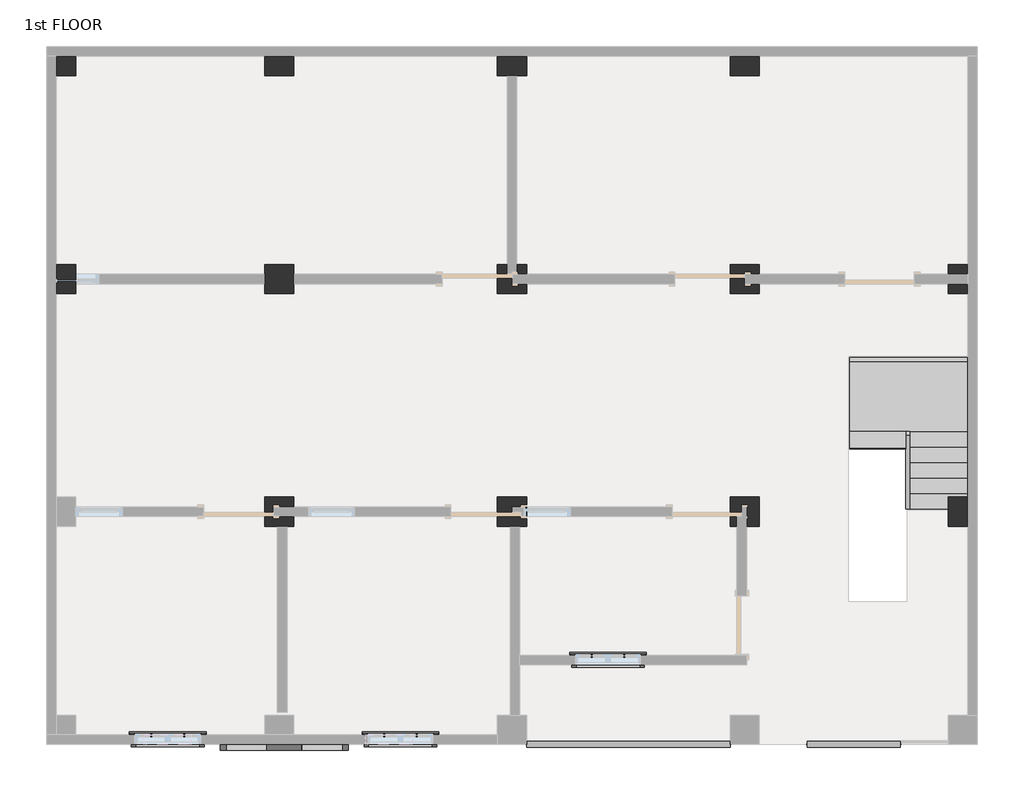
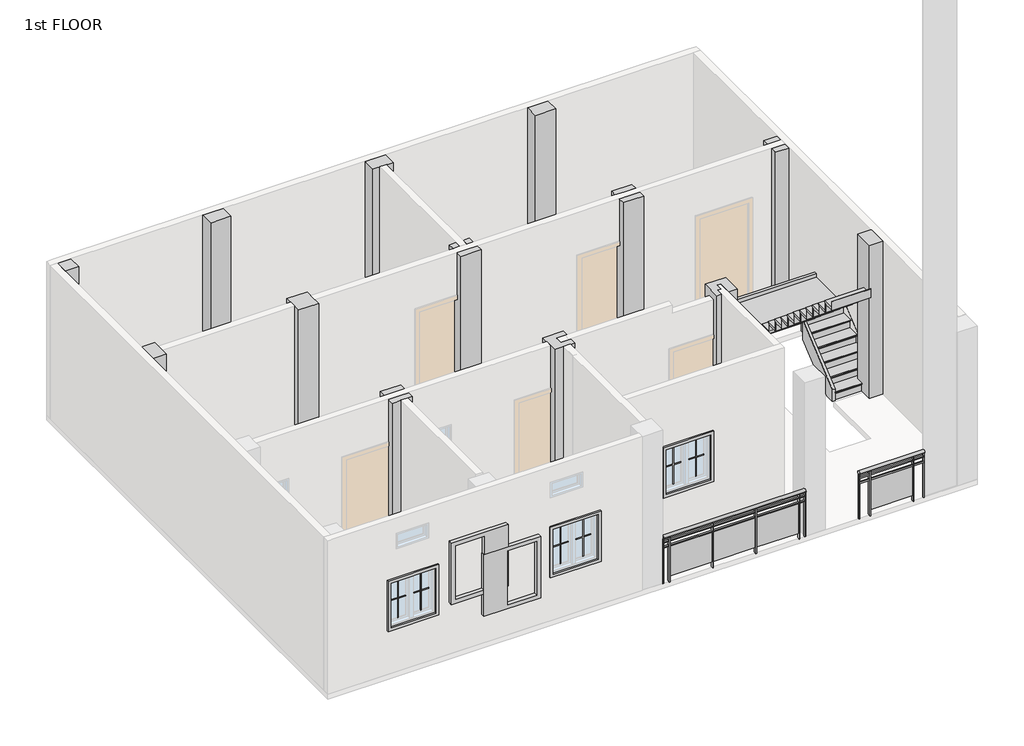
# One storey, part 2 of 2: 13 columns, 12 proxies, 4 members, 2 railings, 1 damper, 1 stair flight.
"""IFC4 building model written with IfcOpenShell, lengths in millimetres."""

from ifc_helpers import new_model, si_unit, point, frame, origin, place, context, project, spatial, polyline, ellipse_curve, trimmed, outline, extrude, faceted_brep, transform, mapped, element, save
from ifc_brep_helpers import plane_surface, extruded_surface, advanced_brep
from components import muntin_pattern_2x2_muntin_pattern_2x2_b3fe6957, muntin_pattern_2x2_muntin_pattern_2x2_3e0ecaf2, trim_window_exterior_flat_with_sill_41619996, trim_window_interior_flat_picture_frame_51c85655, duct_accessories_12_duct_accessories_1_1d6ac5d5, stair_flight_8492ada7

model = new_model("IFC4")

# Units and contexts
model_context = context("Model", 3, world=origin())
ifc_project = project(units=[si_unit("LENGTHUNIT", "METRE", prefix="MILLI")], contexts=[model_context])

# Site, building, storey
site = spatial("IfcSite", under=ifc_project)
building = spatial("IfcBuilding", under=site)
storey = spatial("IfcBuildingStorey", under=building, Name="1st FLOOR", Elevation=3048.0)

# Proxies
placement = place(None, origin())
muntin_pattern_2x2_muntin_pattern_2x2_shape = muntin_pattern_2x2_muntin_pattern_2x2_b3fe6957(model_context)
element("IfcBuildingElementProxy", 1, Name="Muntin Pattern_2x2 : Muntin Pattern_2x2", ObjectType="Muntin Pattern_2x2 : Muntin Pattern_2x2", at=placement, inside=storey, context=model_context, shape_type="MappedRepresentation", body=[
    mapped(muntin_pattern_2x2_muntin_pattern_2x2_shape, transform((-14441.409625, -253.8184478, 4032.25), x_axis=(1.0, 0.0, 0.0), y_axis=(0.0, 1.0, 0.0), z_axis=(0.0, 0.0, 1.0))),
])
element("IfcBuildingElementProxy", 2, Name="Muntin Pattern_2x2 : Muntin Pattern_2x2", ObjectType="Muntin Pattern_2x2 : Muntin Pattern_2x2", at=placement, inside=storey, context=model_context, shape_type="MappedRepresentation", body=[
    mapped(muntin_pattern_2x2_muntin_pattern_2x2_shape, transform((-11393.409625, -253.8184478, 4032.25), x_axis=(1.0, 0.0, 0.0), y_axis=(0.0, 1.0, 0.0), z_axis=(0.0, 0.0, 1.0))),
])
element("IfcBuildingElementProxy", 3, Name="Muntin Pattern_2x2 : Muntin Pattern_2x2", ObjectType="Muntin Pattern_2x2 : Muntin Pattern_2x2", at=placement, inside=storey, context=model_context, shape_type="MappedRepresentation", body=[
    mapped(muntin_pattern_2x2_muntin_pattern_2x2_shape, transform((-8675.609625, 787.5815522, 4032.25), x_axis=(1.0, 0.0, 0.0), y_axis=(0.0, 1.0, 0.0), z_axis=(0.0, 0.0, 1.0))),
])
muntin_pattern_2x2_muntin_pattern_2x2_2_shape = muntin_pattern_2x2_muntin_pattern_2x2_3e0ecaf2(model_context)
element("IfcBuildingElementProxy", 4, Name="Muntin Pattern_2x2 : Muntin Pattern_2x2", ObjectType="Muntin Pattern_2x2 : Muntin Pattern_2x2", at=placement, inside=storey, context=model_context, shape_type="MappedRepresentation", body=[
    mapped(muntin_pattern_2x2_muntin_pattern_2x2_2_shape, transform((-14012.784625, -253.8184478, 4032.25), x_axis=(-1.0, 0.0, 0.0), y_axis=(0.0, -1.0, 0.0), z_axis=(0.0, 0.0, 1.0))),
])
element("IfcBuildingElementProxy", 5, Name="Muntin Pattern_2x2 : Muntin Pattern_2x2", ObjectType="Muntin Pattern_2x2 : Muntin Pattern_2x2", at=placement, inside=storey, context=model_context, shape_type="MappedRepresentation", body=[
    mapped(muntin_pattern_2x2_muntin_pattern_2x2_2_shape, transform((-10964.784625, -253.8184478, 4032.25), x_axis=(-1.0, 0.0, 0.0), y_axis=(0.0, -1.0, 0.0), z_axis=(0.0, 0.0, 1.0))),
])
element("IfcBuildingElementProxy", 6, Name="Muntin Pattern_2x2 : Muntin Pattern_2x2", ObjectType="Muntin Pattern_2x2 : Muntin Pattern_2x2", at=placement, inside=storey, context=model_context, shape_type="MappedRepresentation", body=[
    mapped(muntin_pattern_2x2_muntin_pattern_2x2_2_shape, transform((-8246.984625, 787.5815522, 4032.25), x_axis=(-1.0, 0.0, 0.0), y_axis=(0.0, -1.0, 0.0), z_axis=(0.0, 0.0, 1.0))),
])
trim_window_exterior_flat_with_sill_shape = trim_window_exterior_flat_with_sill_41619996(model_context)
element("IfcBuildingElementProxy", 7, Name="Trim-Window-Exterior-Flat : with Sill", ObjectType="Trim-Window-Exterior-Flat : with Sill", at=placement, inside=storey, context=model_context, shape_type="MappedRepresentation", body=[
    mapped(trim_window_exterior_flat_with_sill_shape, transform((-14227.097125, -244.2934478, 4876.8), x_axis=(-1.0, 0.0, 0.0), y_axis=(0.0, 0.0, 1.0), z_axis=(0.0, 1.0, 0.0))),
])
element("IfcBuildingElementProxy", 8, Name="Trim-Window-Exterior-Flat : with Sill", ObjectType="Trim-Window-Exterior-Flat : with Sill", at=placement, inside=storey, context=model_context, shape_type="MappedRepresentation", body=[
    mapped(trim_window_exterior_flat_with_sill_shape, transform((-11179.097125, -244.2934478, 4876.8), x_axis=(-1.0, 0.0, 0.0), y_axis=(0.0, 0.0, 1.0), z_axis=(0.0, 1.0, 0.0))),
])
element("IfcBuildingElementProxy", 9, Name="Trim-Window-Exterior-Flat : with Sill", ObjectType="Trim-Window-Exterior-Flat : with Sill", at=placement, inside=storey, context=model_context, shape_type="MappedRepresentation", body=[
    mapped(trim_window_exterior_flat_with_sill_shape, transform((-8461.297125, 797.1065522, 4876.8), x_axis=(-1.0, 0.0, 0.0), y_axis=(0.0, 0.0, 1.0), z_axis=(0.0, 1.0, 0.0))),
])
trim_window_interior_flat_picture_frame_shape = trim_window_interior_flat_picture_frame_51c85655(model_context)
element("IfcBuildingElementProxy", 10, Name="Trim-Window-Interior-Flat : Picture Frame", ObjectType="Trim-Window-Interior-Flat : Picture Frame", at=placement, inside=storey, context=model_context, shape_type="MappedRepresentation", body=[
    mapped(trim_window_interior_flat_picture_frame_shape, transform((-14227.097125, -371.2934478, 4876.8), x_axis=(1.0, 0.0, 0.0), y_axis=(0.0, 0.0, 1.0), z_axis=(0.0, -1.0, 0.0))),
])
element("IfcBuildingElementProxy", 11, Name="Trim-Window-Interior-Flat : Picture Frame", ObjectType="Trim-Window-Interior-Flat : Picture Frame", at=placement, inside=storey, context=model_context, shape_type="MappedRepresentation", body=[
    mapped(trim_window_interior_flat_picture_frame_shape, transform((-11179.097125, -371.2934478, 4876.8), x_axis=(1.0, 0.0, 0.0), y_axis=(0.0, 0.0, 1.0), z_axis=(0.0, -1.0, 0.0))),
])
element("IfcBuildingElementProxy", 12, Name="Trim-Window-Interior-Flat : Picture Frame", ObjectType="Trim-Window-Interior-Flat : Picture Frame", at=placement, inside=storey, context=model_context, shape_type="MappedRepresentation", body=[
    mapped(trim_window_interior_flat_picture_frame_shape, transform((-8461.297125, 670.1065522, 4876.8), x_axis=(1.0, 0.0, 0.0), y_axis=(0.0, 0.0, 1.0), z_axis=(0.0, -1.0, 0.0))),
])

# Columns
element("IfcColumn", 13, ObjectType="column family : column family", at=placement, inside=storey, context=model_context, shape_type="Brep", body=[
    faceted_brep([(-15433.597125, 8645.7065522, 3053.0), (-15433.597125, 8391.7065522, 3053.0), (-15687.597125, 8391.7065522, 3053.0), (-15687.597125, 8645.7065522, 3053.0), (-15433.597125, 8391.7065522, 6091.0), (-15433.597125, 8645.7065522, 6091.0), (-15687.597125, 8391.7065522, 6091.0), (-15687.597125, 8645.7065522, 6091.0), (-15687.597125, 8645.7065522, 5943.6)], [[[0, 1, 2, 3]], [[4, 1, 0, 5]], [[1, 4, 6, 2]], [[4, 5, 7, 6]], [[5, 0, 3, 8, 7]], [[3, 2, 6, 7, 8]]]),
])
element("IfcColumn", 14, ObjectType="column family : column family", at=placement, inside=storey, context=model_context, shape_type="SweptSolid", body=[
    extrude(outline(polyline([(-12576.097125, 5915.2065522), (-12576.097125, 5534.2065522), (-12957.097125, 5534.2065522), (-12957.097125, 5915.2065522), (-12576.097125, 5915.2065522)])), frame((0.0, 0.0, 3053.0), z_axis=(0.0, 0.0, 1.0), x_axis=(1.0, 0.0, 0.0)), (0.0, 0.0, 1.0), 3038.0),
])
element("IfcColumn", 15, ObjectType="column family : column family", at=placement, inside=storey, context=model_context, shape_type="Brep", body=[
    faceted_brep([(-9655.097125, 5915.2065522, 3053.0), (-9528.097125, 5915.2065522, 3053.0), (-9528.097125, 5788.2065522, 3053.0), (-9655.097125, 5788.2065522, 3053.0), (-9528.097125, 5915.2065522, 6091.0), (-9655.097125, 5915.2065522, 6091.0), (-9655.097125, 5788.2065522, 6091.0), (-9528.097125, 5788.2065522, 6091.0), (-9655.097125, 5788.2065522, 5943.6), (-9655.097125, 5915.2065522, 5943.6), (-9528.097125, 5788.2065522, 5943.6)], [[[0, 1, 2, 3]], [[4, 5, 6, 7]], [[0, 3, 8, 6, 5, 9]], [[4, 1, 0, 9, 5]], [[3, 2, 10, 7, 6, 8]], [[1, 4, 7, 10, 2]]]),
    faceted_brep([(-9528.097125, 5534.2065522, 6091.0), (-9528.097125, 5534.2065522, 3053.0), (-9528.097125, 5661.2065522, 3053.0), (-9528.097125, 5661.2065522, 5943.6), (-9528.097125, 5661.2065522, 6091.0), (-9909.097125, 5534.2065522, 3053.0), (-9909.097125, 5534.2065522, 6091.0), (-9909.097125, 5915.2065522, 3053.0), (-9909.097125, 5661.2065522, 6091.0), (-9909.097125, 5661.2065522, 5181.6), (-9909.097125, 5788.2065522, 5181.6), (-9909.097125, 5788.2065522, 6091.0), (-9909.097125, 5915.2065522, 6091.0), (-9782.097125, 5915.2065522, 6091.0), (-9782.097125, 5915.2065522, 5943.6), (-9782.097125, 5915.2065522, 3053.0), (-9782.097125, 5788.2065522, 3053.0), (-9782.097125, 5788.2065522, 6091.0), (-9782.097125, 5788.2065522, 5943.6), (-9782.097125, 5788.2065522, 5181.6), (-9718.597125, 5788.2065522, 3053.0), (-9718.597125, 5788.2065522, 5181.6), (-9718.597125, 5661.2065522, 3053.0), (-9718.597125, 5661.2065522, 5181.6), (-9718.597125, 5661.2065522, 6091.0)], [[[0, 1, 2, 3, 4]], [[5, 1, 0, 6]], [[7, 5, 6, 8, 9, 10, 11, 12]], [[7, 12, 13, 14, 15]], [[16, 15, 14, 13, 17, 18, 19]], [[20, 16, 19, 21]], [[2, 22, 23, 9, 8, 24, 4, 3]], [[1, 5, 7, 15, 16, 20, 22, 2]], [[6, 0, 4, 24, 8]], [[13, 12, 11, 17]], [[11, 10, 19, 18, 17]], [[21, 23, 22, 20]], [[23, 21, 19, 10, 9]]]),
])
element("IfcColumn", 16, ObjectType="column family : column family", at=placement, inside=storey, context=model_context, shape_type="Brep", body=[
    faceted_brep([(-6480.097125, 5534.2065522, 3053.0), (-6861.097125, 5534.2065522, 3053.0), (-6861.097125, 5915.2065522, 3053.0), (-6480.097125, 5915.2065522, 3053.0), (-6480.097125, 5788.2065522, 3053.0), (-6670.597125, 5788.2065522, 3053.0), (-6670.597125, 5661.2065522, 3053.0), (-6480.097125, 5661.2065522, 3053.0), (-6480.097125, 5534.2065522, 6091.0), (-6480.097125, 5661.2065522, 5943.6), (-6480.097125, 5661.2065522, 6091.0), (-6861.097125, 5534.2065522, 6091.0), (-6861.097125, 5661.2065522, 6091.0), (-6861.097125, 5661.2065522, 5181.6), (-6861.097125, 5788.2065522, 5181.6), (-6861.097125, 5788.2065522, 6091.0), (-6861.097125, 5915.2065522, 6091.0), (-6480.097125, 5915.2065522, 6091.0), (-6670.597125, 5661.2065522, 6091.0), (-6670.597125, 5661.2065522, 5181.6), (-6480.097125, 5788.2065522, 5943.6), (-6480.097125, 5788.2065522, 6091.0), (-6670.597125, 5788.2065522, 6091.0), (-6670.597125, 5788.2065522, 5181.6)], [[[0, 1, 2, 3, 4, 5, 6, 7]], [[8, 0, 7, 9, 10]], [[1, 0, 8, 11]], [[2, 1, 11, 12, 13, 14, 15, 16]], [[3, 2, 16, 17]], [[11, 8, 10, 18, 12]], [[7, 6, 19, 13, 12, 18, 10, 9]], [[5, 4, 20, 21, 22, 15, 14, 23]], [[3, 17, 21, 20, 4]], [[17, 16, 15, 22, 21]], [[23, 19, 6, 5]], [[19, 23, 14, 13]]]),
])
element("IfcColumn", 17, ObjectType="column family : column family", at=placement, inside=storey, context=model_context, shape_type="Brep", body=[
    faceted_brep([(-6480.097125, 2867.2065522, 3053.0), (-6480.097125, 2486.2065522, 3053.0), (-6645.197125, 2486.2065522, 3053.0), (-6645.197125, 2740.2065522, 3053.0), (-6708.697125, 2740.2065522, 3053.0), (-6708.697125, 2613.2065522, 3053.0), (-6772.197125, 2613.2065522, 3053.0), (-6772.197125, 2486.2065522, 3053.0), (-6861.097125, 2486.2065522, 3053.0), (-6861.097125, 2867.2065522, 3053.0), (-6480.097125, 2867.2065522, 6091.0), (-6480.097125, 2486.2065522, 6091.0), (-6861.097125, 2486.2065522, 6091.0), (-6772.197125, 2486.2065522, 5943.6), (-6772.197125, 2486.2065522, 6091.0), (-6861.097125, 2867.2065522, 6091.0), (-6861.097125, 2613.2065522, 5943.6), (-6861.097125, 2613.2065522, 5181.6), (-6861.097125, 2740.2065522, 5181.6), (-6861.097125, 2740.2065522, 5943.6), (-6772.197125, 2613.2065522, 6091.0), (-6708.697125, 2613.2065522, 6091.0), (-6708.697125, 2740.2065522, 6091.0), (-6645.197125, 2740.2065522, 6091.0), (-6645.197125, 2613.2065522, 6091.0), (-6645.197125, 2486.2065522, 6091.0), (-6772.197125, 2613.2065522, 5943.6), (-6772.197125, 2613.2065522, 5181.6), (-6772.197125, 2740.2065522, 5181.6), (-6772.197125, 2740.2065522, 5943.6), (-6645.197125, 2486.2065522, 5943.6), (-6708.697125, 2613.2065522, 5181.6), (-6708.697125, 2740.2065522, 5181.6), (-6708.697125, 2740.2065522, 5943.6), (-6708.697125, 2613.2065522, 5943.6)], [[[0, 1, 2, 3, 4, 5, 6, 7, 8, 9]], [[1, 0, 10, 11]], [[12, 8, 7, 13, 14]], [[9, 8, 12, 15], [16, 17, 18, 19]], [[0, 9, 15, 10]], [[11, 10, 15, 12, 14, 20, 21, 22, 23, 24, 25]], [[17, 16, 26, 27]], [[19, 18, 28, 29]], [[3, 2, 30, 25, 24, 23]], [[20, 14, 13, 7, 6, 27, 26]], [[1, 11, 25, 30, 2]], [[17, 27, 28, 18]], [[31, 27, 6, 5]], [[27, 31, 32, 28]], [[31, 5, 4, 32]], [[26, 16, 19, 29]], [[28, 32, 4, 3, 23, 22, 33, 29]], [[26, 34, 21, 20]], [[29, 33, 34, 26]], [[34, 33, 22, 21]]]),
])
element("IfcColumn", 18, ObjectType="column family : column family", at=placement, inside=storey, context=model_context, shape_type="Brep", body=[
    faceted_brep([(-9528.097125, 2486.2065522, 3053.0), (-9909.097125, 2486.2065522, 3053.0), (-9909.097125, 2867.2065522, 3053.0), (-9528.097125, 2867.2065522, 3053.0), (-9528.097125, 2740.2065522, 3053.0), (-9566.197125, 2740.2065522, 3053.0), (-9718.597125, 2740.2065522, 3053.0), (-9718.597125, 2613.2065522, 3053.0), (-9566.197125, 2613.2065522, 3053.0), (-9528.097125, 2613.2065522, 3053.0), (-9528.097125, 2486.2065522, 6091.0), (-9528.097125, 2613.2065522, 3352.8), (-9528.097125, 2740.2065522, 3352.8), (-9528.097125, 2867.2065522, 6091.0), (-9528.097125, 2740.2065522, 6091.0), (-9528.097125, 2740.2065522, 5943.6), (-9528.097125, 2740.2065522, 5181.6), (-9528.097125, 2613.2065522, 5181.6), (-9528.097125, 2613.2065522, 5943.6), (-9528.097125, 2613.2065522, 6091.0), (-9909.097125, 2486.2065522, 6091.0), (-9909.097125, 2867.2065522, 6091.0), (-9566.197125, 2613.2065522, 6091.0), (-9718.597125, 2613.2065522, 6091.0), (-9718.597125, 2740.2065522, 6091.0), (-9566.197125, 2740.2065522, 6091.0), (-9718.597125, 2613.2065522, 5943.6), (-9566.197125, 2613.2065522, 5181.6), (-9566.197125, 2613.2065522, 3352.8), (-9566.197125, 2740.2065522, 3352.8), (-9566.197125, 2740.2065522, 5181.6), (-9718.597125, 2740.2065522, 5943.6)], [[[0, 1, 2, 3, 4, 5, 6, 7, 8, 9]], [[10, 0, 9, 11, 12, 4, 3, 13, 14, 15, 16, 17, 18, 19]], [[1, 0, 10, 20]], [[2, 1, 20, 21]], [[3, 2, 21, 13]], [[20, 10, 19, 22, 23, 24, 25, 14, 13, 21]], [[11, 9, 8, 7, 26, 23, 22, 19, 18, 17, 27, 28]], [[4, 12, 29, 30, 16, 15, 14, 25, 24, 31, 6, 5]], [[7, 6, 31, 24, 23, 26]], [[28, 27, 30, 29]], [[28, 29, 12, 11]], [[30, 27, 17, 16]]]),
])
element("IfcColumn", 19, ObjectType="column family : column family", at=placement, inside=storey, context=model_context, shape_type="Brep", body=[
    faceted_brep([(-12576.097125, 2486.2065522, 3053.0), (-12957.097125, 2486.2065522, 3053.0), (-12957.097125, 2867.2065522, 3053.0), (-12576.097125, 2867.2065522, 3053.0), (-12576.097125, 2740.2065522, 3053.0), (-12842.797125, 2740.2065522, 3053.0), (-12842.797125, 2613.2065522, 3053.0), (-12576.097125, 2613.2065522, 3053.0), (-12576.097125, 2486.2065522, 6091.0), (-12576.097125, 2613.2065522, 5943.6), (-12576.097125, 2613.2065522, 6091.0), (-12957.097125, 2486.2065522, 6091.0), (-12957.097125, 2613.2065522, 6091.0), (-12957.097125, 2613.2065522, 5181.6), (-12957.097125, 2740.2065522, 5181.6), (-12957.097125, 2740.2065522, 6091.0), (-12957.097125, 2867.2065522, 6091.0), (-12576.097125, 2867.2065522, 6091.0), (-12842.797125, 2613.2065522, 6091.0), (-12842.797125, 2613.2065522, 5181.6), (-12576.097125, 2740.2065522, 5943.6), (-12576.097125, 2740.2065522, 6091.0), (-12842.797125, 2740.2065522, 6091.0), (-12842.797125, 2740.2065522, 5181.6)], [[[0, 1, 2, 3, 4, 5, 6, 7]], [[8, 0, 7, 9, 10]], [[1, 0, 8, 11]], [[2, 1, 11, 12, 13, 14, 15, 16]], [[3, 2, 16, 17]], [[11, 8, 10, 18, 12]], [[7, 6, 19, 13, 12, 18, 10, 9]], [[5, 4, 20, 21, 22, 15, 14, 23]], [[3, 17, 21, 20, 4]], [[17, 16, 15, 22, 21]], [[19, 23, 14, 13]], [[23, 19, 6, 5]]]),
])
element("IfcColumn", 20, ObjectType="column family : column family", at=placement, inside=storey, context=model_context, shape_type="SweptSolid", body=[
    extrude(outline(polyline([(-12576.097125, 8391.7065522), (-12957.097125, 8391.7065522), (-12957.097125, 8645.7065522), (-12576.097125, 8645.7065522), (-12576.097125, 8391.7065522)])), frame((0.0, 0.0, 3053.0), z_axis=(0.0, 0.0, 1.0), x_axis=(1.0, 0.0, 0.0)), (0.0, 0.0, 1.0), 3038.0),
])
element("IfcColumn", 21, ObjectType="column family : column family", at=placement, inside=storey, context=model_context, shape_type="SweptSolid", body=[
    extrude(outline(polyline([(-9528.097125, 8391.7065522), (-9909.097125, 8391.7065522), (-9909.097125, 8645.7065522), (-9528.097125, 8645.7065522), (-9528.097125, 8391.7065522)])), frame((0.0, 0.0, 3053.0), z_axis=(0.0, 0.0, 1.0), x_axis=(1.0, 0.0, 0.0)), (0.0, 0.0, 1.0), 3038.0),
])
element("IfcColumn", 22, ObjectType="column family : column family", at=placement, inside=storey, context=model_context, shape_type="SweptSolid", body=[
    extrude(outline(polyline([(-6480.097125, 8391.7065522), (-6861.097125, 8391.7065522), (-6861.097125, 8645.7065522), (-6480.097125, 8645.7065522), (-6480.097125, 8391.7065522)])), frame((0.0, 0.0, 3053.0), z_axis=(0.0, 0.0, 1.0), x_axis=(1.0, 0.0, 0.0)), (0.0, 0.0, 1.0), 3038.0),
])
element("IfcColumn", 23, ObjectType="column family : column family", at=placement, inside=storey, context=model_context, shape_type="Brep", body=[
    faceted_brep([(-4003.597125, 5915.2065522, 3053.0), (-3749.597125, 5915.2065522, 3053.0), (-3749.597125, 5788.2065522, 3053.0), (-4003.597125, 5788.2065522, 3053.0), (-4003.597125, 5915.2065522, 6091.0), (-4003.597125, 5788.2065522, 5943.6), (-4003.597125, 5788.2065522, 6091.0), (-3749.597125, 5915.2065522, 6091.0), (-3749.597125, 5788.2065522, 6091.0), (-3749.597125, 5788.2065522, 5943.6)], [[[0, 1, 2, 3]], [[4, 0, 3, 5, 6]], [[0, 4, 7, 1]], [[1, 7, 8, 9, 2]], [[3, 2, 9, 8, 6, 5]], [[7, 4, 6, 8]]]),
    faceted_brep([(-4003.597125, 5534.2065522, 6091.0), (-4003.597125, 5534.2065522, 3053.0), (-3749.597125, 5534.2065522, 3053.0), (-3749.597125, 5534.2065522, 6091.0), (-3749.597125, 5661.2065522, 6091.0), (-4003.597125, 5661.2065522, 6091.0), (-3749.597125, 5661.2065522, 3053.0), (-4003.597125, 5661.2065522, 3053.0), (-4003.597125, 5661.2065522, 5943.6), (-3749.597125, 5661.2065522, 5943.6)], [[[0, 1, 2, 3]], [[0, 3, 4, 5]], [[6, 7, 8, 5, 4, 9]], [[2, 1, 7, 6]], [[3, 2, 6, 9, 4]], [[1, 0, 5, 8, 7]]]),
])
element("IfcColumn", 24, ObjectType="column family : column family", at=placement, inside=storey, context=model_context, shape_type="SweptSolid", body=[
    extrude(outline(polyline([(-4003.597125, 2486.2065522), (-4003.597125, 2867.2065522), (-3749.597125, 2867.2065522), (-3749.597125, 2486.2065522), (-4003.597125, 2486.2065522)])), frame((0.0, 0.0, 3053.0), z_axis=(0.0, 0.0, 1.0), x_axis=(1.0, 0.0, 0.0)), (0.0, 0.0, 1.0), 3038.0),
])
element("IfcColumn", 25, ObjectType="column family : column family", at=placement, inside=storey, context=model_context, shape_type="SweptSolid", body=[
    extrude(outline(polyline([(-15433.597125, 5915.2065522), (-15433.597125, 5534.2065522), (-15687.597125, 5534.2065522), (-15687.597125, 5915.2065522), (-15433.597125, 5915.2065522)])), frame((0.0, 0.0, 3053.0), z_axis=(0.0, 0.0, 1.0), x_axis=(1.0, 0.0, 0.0)), (0.0, 0.0, 1.0), 3038.0),
])

# Damper
duct_accessories_12_duct_accessories_1_shape = duct_accessories_12_duct_accessories_1_1d6ac5d5(model_context)
element("IfcDamper", 26, ObjectType="Duct Accessories 12 : Duct Accessories 1", at=placement, inside=storey, context=model_context, shape_type="MappedRepresentation", body=[
    mapped(duct_accessories_12_duct_accessories_1_shape, transform((0.0, 0.0, 0.0), x_axis=(1.0, 0.0, 0.0), y_axis=(0.0, 1.0, 0.0), z_axis=(0.0, 0.0, 1.0))),
])

# Members
element("IfcMember", 27, ObjectType="Stringer - 2\" Width", at=placement, inside=storey, context=model_context, shape_type="SweptSolid", body=[
    extrude(outline(polyline([(2714.6319226, 3048.0), (2714.6319226, 3284.8438745), (3679.8319226, 4089.1772078), (3679.8319226, 3692.4165243), (2906.5320935, 3048.0), (2714.6319226, 3048.0)])), frame((-4563.0136682, 0.0, 0.0), z_axis=(1.0, 0.0, 0.0), x_axis=(0.0, 1.0, 0.0)), (0.0, 0.0, 1.0), 50.8),
])
element("IfcMember", 28, ObjectType="Stringer - 2\" Width", at=placement, inside=storey, context=model_context, shape_type="SweptSolid", body=[
    extrude(outline(polyline([(-4512.2136682, 3730.6319226), (-4512.2136682, 3679.8319226), (-4563.0136682, 3679.8319226), (-4563.0136682, 3730.6319226), (-4512.2136682, 3730.6319226)])), frame((0.0, 0.0, 3835.4), z_axis=(0.0, 0.0, 1.0), x_axis=(1.0, 0.0, 0.0)), (0.0, 0.0, 1.0), 304.8),
])
element("IfcMember", 29, ObjectType="Stringer - 2\" Width", at=placement, inside=storey, context=model_context, shape_type="SweptSolid", body=[
    extrude(outline(polyline([(2714.6319226, 3048.0), (2714.6319226, 3284.8438745), (3741.0592732, 4140.2), (4217.1720935, 4140.2), (2906.5320935, 3048.0), (2714.6319226, 3048.0)])), frame((-3749.597125, 0.0, 0.0), z_axis=(1.0, 0.0, 0.0), x_axis=(0.0, 1.0, 0.0)), (0.0, 0.0, 1.0), 50.8),
])
element("IfcMember", 30, ObjectType="Stringer - 2\" Width", at=placement, inside=storey, context=model_context, shape_type="SweptSolid", body=[
    extrude(outline(polyline([(-3698.797125, 4695.8319226), (-3698.797125, 4645.0319226), (-5295.0246464, 4645.0319226), (-5295.0246464, 4695.8319226), (-3698.797125, 4695.8319226)])), frame((0.0, 0.0, 3835.4), z_axis=(0.0, 0.0, 1.0), x_axis=(1.0, 0.0, 0.0)), (0.0, 0.0, 1.0), 304.8),
])

# Railings
element("IfcRailing", 31, ObjectType="Glass Panel - Bottom Fill", at=placement, inside=storey, context=model_context, shape_type="SolidModel", body=[
    advanced_brep(
    [(-5851.447125, -333.1934478, 3962.4), (-5851.447125, -409.3934478, 3962.4), (-4632.247125, -333.1934478, 3962.4), (-4632.247125, -409.3934478, 3962.4)],
    [
        (0, 1, ellipse_curve(frame((-5851.447125, -371.2934478, 3962.4), z_axis=(-1.0, 0.0, 0.0), x_axis=(0.0, -1.0, 0.0)), 38.1, 28.575)),
        (1, 0, ellipse_curve(frame((-5851.447125, -371.2934478, 3962.4), z_axis=(-1.0, 0.0, 0.0), x_axis=(0.0, -1.0, 0.0)), 38.1, 28.575)),
        (2, 3, ellipse_curve(frame((-4632.247125, -371.2934478, 3962.4), z_axis=(1.0, 0.0, 0.0), x_axis=(0.0, -1.0, 0.0)), 38.1, 28.575)),
        (3, 2, ellipse_curve(frame((-4632.247125, -371.2934478, 3962.4), z_axis=(1.0, 0.0, 0.0), x_axis=(0.0, -1.0, 0.0)), 38.1, 28.575)),
        (0, 2),
        (3, 1),
    ],
    [
        plane_surface(frame((-5851.447125, -371.2934478, 3962.4), z_axis=(-1.0, 0.0, 0.0), x_axis=(0.0, 1.0, 0.0))),
        plane_surface(frame((-4632.247125, -371.2934478, 3962.4), z_axis=(1.0, 0.0, 0.0), x_axis=(0.0, 1.0, 0.0))),
        extruded_surface(trimmed(ellipse_curve(frame((-4632.247125, -371.2934478, 3962.4), z_axis=(-1.0, 0.0, 0.0), x_axis=(0.0, -1.0, 0.0)), 38.1, 28.575), [point((-4632.247125, -333.1934478, 3962.4))], [point((-4632.247125, -409.3934478, 3962.4))], True, "CARTESIAN"), (-1219.1999999999998, 0.0, 0.0), 1219.1999999999998),
        extruded_surface(trimmed(ellipse_curve(frame((-4632.247125, -371.2934478, 3962.4), z_axis=(-1.0, 0.0, 0.0), x_axis=(0.0, -1.0, 0.0)), 38.1, 28.575), [point((-4632.247125, -409.3934478, 3962.4))], [point((-4632.247125, -333.1934478, 3962.4))], True, "CARTESIAN"), (-1219.1999999999998, 0.0, 0.0), 1219.1999999999998),
    ],
    [
        (0, [[1, 2]]),
        (1, [[3, 4]]),
        (2, [[-1, 5, -4, 6]]),
        (3, [[-2, -6, -3, -5]]),
    ],
),
    extrude(outline(polyline([(-5851.447125, -383.9934478), (-5851.447125, -358.5934478), (-4632.247125, -358.5934478), (-4632.247125, -383.9934478), (-5851.447125, -383.9934478)])), frame((0.0, 0.0, 3848.1), z_axis=(0.0, 0.0, 1.0), x_axis=(1.0, 0.0, 0.0)), (0.0, 0.0, 1.0), 25.4),
    extrude(outline(polyline([(-5851.447125, -383.9934478), (-5851.447125, -358.5934478), (-4632.247125, -358.5934478), (-4632.247125, -383.9934478), (-5851.447125, -383.9934478)])), frame((0.0, 0.0, 3746.5), z_axis=(0.0, 0.0, 1.0), x_axis=(1.0, 0.0, 0.0)), (0.0, 0.0, 1.0), 25.4),
    extrude(outline(polyline([(-4841.797125, -396.6934478), (-4841.797125, -345.8934478), (-4829.097125, -345.8934478), (-4829.097125, -396.6934478), (-4841.797125, -396.6934478)])), frame((0.0, 0.0, 3048.0), z_axis=(0.0, 0.0, 1.0), x_axis=(1.0, 0.0, 0.0)), (0.0, 0.0, 1.0), 885.6788223),
    extrude(outline(polyline([(-5648.247125, -364.7582908), (-4835.447125, -364.7582908), (-4835.447125, -371.1082908), (-5648.247125, -371.1082908), (-5648.247125, -364.7582908)])), frame((0.0, 0.0, 3149.6), z_axis=(0.0, 0.0, 1.0), x_axis=(1.0, 0.0, 0.0)), (0.0, 0.0, 1.0), 596.9),
    extrude(outline(polyline([(-5654.597125, -396.6934478), (-5654.597125, -345.8934478), (-5641.897125, -345.8934478), (-5641.897125, -396.6934478), (-5654.597125, -396.6934478)])), frame((0.0, 0.0, 3048.0), z_axis=(0.0, 0.0, 1.0), x_axis=(1.0, 0.0, 0.0)), (0.0, 0.0, 1.0), 885.6788223),
    extrude(outline(polyline([(-4644.947125, -380.8184478), (-4644.947125, -361.7684478), (-4625.897125, -361.7684478), (-4625.897125, -380.8184478), (-4644.947125, -380.8184478)])), frame((0.0, 0.0, 3048.0), z_axis=(0.0, 0.0, 1.0), x_axis=(1.0, 0.0, 0.0)), (0.0, 0.0, 1.0), 885.6788223),
    extrude(outline(polyline([(-5857.797125, -380.8184478), (-5857.797125, -361.7684478), (-5838.747125, -361.7684478), (-5838.747125, -380.8184478), (-5857.797125, -380.8184478)])), frame((0.0, 0.0, 3048.0), z_axis=(0.0, 0.0, 1.0), x_axis=(1.0, 0.0, 0.0)), (0.0, 0.0, 1.0), 885.6788223),
])
element("IfcRailing", 32, ObjectType="Glass Panel - Bottom Fill", at=placement, inside=storey, context=model_context, shape_type="SolidModel", body=[
    advanced_brep(
    [(-9528.097125, -333.1934478, 3962.4), (-9528.097125, -409.3934478, 3962.4), (-6861.097125, -333.1934478, 3962.4), (-6861.097125, -409.3934478, 3962.4)],
    [
        (0, 1, ellipse_curve(frame((-9528.097125, -371.2934478, 3962.4), z_axis=(-1.0, 0.0, 0.0), x_axis=(0.0, -1.0, 0.0)), 38.1, 28.575)),
        (1, 0, ellipse_curve(frame((-9528.097125, -371.2934478, 3962.4), z_axis=(-1.0, 0.0, 0.0), x_axis=(0.0, -1.0, 0.0)), 38.1, 28.575)),
        (2, 3, ellipse_curve(frame((-6861.097125, -371.2934478, 3962.4), z_axis=(1.0, 0.0, 0.0), x_axis=(0.0, -1.0, 0.0)), 38.1, 28.575)),
        (3, 2, ellipse_curve(frame((-6861.097125, -371.2934478, 3962.4), z_axis=(1.0, 0.0, 0.0), x_axis=(0.0, -1.0, 0.0)), 38.1, 28.575)),
        (0, 2),
        (3, 1),
    ],
    [
        plane_surface(frame((-9528.097125, -371.2934478, 3962.4), z_axis=(-1.0, 0.0, 0.0), x_axis=(0.0, 1.0, 0.0))),
        plane_surface(frame((-6861.097125, -371.2934478, 3962.4), z_axis=(1.0, 0.0, 0.0), x_axis=(0.0, 1.0, 0.0))),
        extruded_surface(trimmed(ellipse_curve(frame((-6861.097125, -371.2934478, 3962.4), z_axis=(-1.0, 0.0, 0.0), x_axis=(0.0, -1.0, 0.0)), 38.1, 28.575), [point((-6861.097125, -333.1934478, 3962.4))], [point((-6861.097125, -409.3934478, 3962.4))], True, "CARTESIAN"), (-2667.0, 0.0, 0.0), 2667.0),
        extruded_surface(trimmed(ellipse_curve(frame((-6861.097125, -371.2934478, 3962.4), z_axis=(-1.0, 0.0, 0.0), x_axis=(0.0, -1.0, 0.0)), 38.1, 28.575), [point((-6861.097125, -409.3934478, 3962.4))], [point((-6861.097125, -333.1934478, 3962.4))], True, "CARTESIAN"), (-2667.0, 0.0, 0.0), 2667.0),
    ],
    [
        (0, [[1, 2]]),
        (1, [[3, 4]]),
        (2, [[-1, 5, -4, 6]]),
        (3, [[-2, -6, -3, -5]]),
    ],
),
    extrude(outline(polyline([(-9528.097125, -383.9934478), (-9528.097125, -358.5934478), (-6861.097125, -358.5934478), (-6861.097125, -383.9934478), (-9528.097125, -383.9934478)])), frame((0.0, 0.0, 3848.1), z_axis=(0.0, 0.0, 1.0), x_axis=(1.0, 0.0, 0.0)), (0.0, 0.0, 1.0), 25.4),
    extrude(outline(polyline([(-9528.097125, -383.9934478), (-9528.097125, -358.5934478), (-6861.097125, -358.5934478), (-6861.097125, -383.9934478), (-9528.097125, -383.9934478)])), frame((0.0, 0.0, 3746.5), z_axis=(0.0, 0.0, 1.0), x_axis=(1.0, 0.0, 0.0)), (0.0, 0.0, 1.0), 25.4),
    extrude(outline(polyline([(-6981.747125, -396.6934478), (-6981.747125, -345.8934478), (-6969.047125, -345.8934478), (-6969.047125, -396.6934478), (-6981.747125, -396.6934478)])), frame((0.0, 0.0, 3048.0), z_axis=(0.0, 0.0, 1.0), x_axis=(1.0, 0.0, 0.0)), (0.0, 0.0, 1.0), 885.6788223),
    extrude(outline(polyline([(-7788.197125, -364.7582908), (-6975.397125, -364.7582908), (-6975.397125, -371.1082908), (-7788.197125, -371.1082908), (-7788.197125, -364.7582908)])), frame((0.0, 0.0, 3149.6), z_axis=(0.0, 0.0, 1.0), x_axis=(1.0, 0.0, 0.0)), (0.0, 0.0, 1.0), 596.9),
    extrude(outline(polyline([(-7794.547125, -396.6934478), (-7794.547125, -345.8934478), (-7781.847125, -345.8934478), (-7781.847125, -396.6934478), (-7794.547125, -396.6934478)])), frame((0.0, 0.0, 3048.0), z_axis=(0.0, 0.0, 1.0), x_axis=(1.0, 0.0, 0.0)), (0.0, 0.0, 1.0), 885.6788223),
    extrude(outline(polyline([(-8600.997125, -364.7582908), (-7788.197125, -364.7582908), (-7788.197125, -371.1082908), (-8600.997125, -371.1082908), (-8600.997125, -364.7582908)])), frame((0.0, 0.0, 3149.6), z_axis=(0.0, 0.0, 1.0), x_axis=(1.0, 0.0, 0.0)), (0.0, 0.0, 1.0), 596.9),
    extrude(outline(polyline([(-8607.347125, -396.6934478), (-8607.347125, -345.8934478), (-8594.647125, -345.8934478), (-8594.647125, -396.6934478), (-8607.347125, -396.6934478)])), frame((0.0, 0.0, 3048.0), z_axis=(0.0, 0.0, 1.0), x_axis=(1.0, 0.0, 0.0)), (0.0, 0.0, 1.0), 885.6788223),
    extrude(outline(polyline([(-9413.797125, -364.7582908), (-8600.997125, -364.7582908), (-8600.997125, -371.1082908), (-9413.797125, -371.1082908), (-9413.797125, -364.7582908)])), frame((0.0, 0.0, 3149.6), z_axis=(0.0, 0.0, 1.0), x_axis=(1.0, 0.0, 0.0)), (0.0, 0.0, 1.0), 596.9),
    extrude(outline(polyline([(-9420.147125, -396.6934478), (-9420.147125, -345.8934478), (-9407.447125, -345.8934478), (-9407.447125, -396.6934478), (-9420.147125, -396.6934478)])), frame((0.0, 0.0, 3048.0), z_axis=(0.0, 0.0, 1.0), x_axis=(1.0, 0.0, 0.0)), (0.0, 0.0, 1.0), 885.6788223),
    extrude(outline(polyline([(-6873.797125, -380.8184478), (-6873.797125, -361.7684478), (-6854.747125, -361.7684478), (-6854.747125, -380.8184478), (-6873.797125, -380.8184478)])), frame((0.0, 0.0, 3048.0), z_axis=(0.0, 0.0, 1.0), x_axis=(1.0, 0.0, 0.0)), (0.0, 0.0, 1.0), 885.6788223),
    extrude(outline(polyline([(-9534.447125, -380.8184478), (-9534.447125, -361.7684478), (-9515.397125, -361.7684478), (-9515.397125, -380.8184478), (-9534.447125, -380.8184478)])), frame((0.0, 0.0, 3048.0), z_axis=(0.0, 0.0, 1.0), x_axis=(1.0, 0.0, 0.0)), (0.0, 0.0, 1.0), 885.6788223),
])

# Stair flight
stair_flight_shape = stair_flight_8492ada7(model_context)
element("IfcStairFlight", 33, ObjectType="2\" Tread 1\" Nosing 1/4\" Riser", at=placement, inside=storey, context=model_context, shape_type="MappedRepresentation", body=[
    mapped(stair_flight_shape, transform((0.0, 0.0, 0.0), x_axis=(1.0, 0.0, 0.0), y_axis=(0.0, 1.0, 0.0), z_axis=(0.0, 0.0, 1.0))),
])

save(model, "model.ifc")

# Revit data of these elements
# Type "Muntin Pattern_2x2 : Muntin Pattern_2x2"
#   Width [instance default] = 4' - 0"
#   Thickness = 0' - 0 1/2"
#   Height [instance default] = 4' - 0"
#   Distance = 0' - 0 3/4"
#   Interior Material [instance default] = none
#   Exterior Material [instance default] = none
#   Default Elevation = 0
# Type "Trim-Window-Exterior-Flat : with Sill"
#   Trim Width = 0' - 2 1/4"
#   Trim Thickness_Picture Frame = 0' - 1 1/4"
#   Trim Thickness_with Sill = 0' - 0 3/4"
#   Sill Thickness = 0' - 1 1/4"
#   Opening Width [instance default] = 2' - 0"
#   Opening Height [instance default] = 3' - 0"
#   Default Elevation = 4' - 0"
#   Sill = yes
#   Picture Frame = no
#   Trim Material [instance default] = none
# Type "Trim-Window-Interior-Flat : Picture Frame"
#   Trim Thickness_Picture Frame = 0' - 1 1/4"
#   Trim Width = 0' - 2 1/4"
#   Trim Thickness_with Sill = 0' - 0 3/4"
#   Sill Thickness = 0' - 1 1/4"
#   Opening Width [instance default] = 2' - 0"
#   Opening Height [instance default] = 3' - 0"
#   Default Elevation = 4' - 0"
#   Sill = no
#   Picture Frame = yes
#   Trim Material [instance default] = none
# Type "column family : column family"
#   w2 [instance default] = 0' - 9.88189"
#   w1 [instance default] = 0' - 9.01575"
#   Depth = 1' - 11.62205"
#   Width = 1' - 11.62205"
# Type "Glass Panel - Bottom Fill"
#   Assembly Code = "C2010400"
#   built-in parameter 1008612 = 0.0416667 (stored number, unit not read)
#   built-in parameter 1008611 = 0.0416667 (stored number, unit not read)
#   built-in parameter 1008609 = 0.333333 (stored number, unit not read)
#   built-in parameter 1008604 = 0.166667 (stored number, unit not read)
#   built-in parameter 1008603 = 0.166667 (stored number, unit not read)
#   Railing Height = 3' - 0"
#   built-in parameter 1008630 = 2
#   built-in parameter 1008610 = 2
#   built-in parameter 1008618 = Baluster - Square : 3/4"
# Elements 1, 2, 3, 4, 5, 6 (IfcBuildingElementProxy, "Muntin Pattern_2x2 : Muntin Pattern_2x2")
#   Width = 0' - 11 5/8"
#   Height = 2' - 6 1/2"
#   Interior Material = Wood - Stained
#   Exterior Material = Clad - White
#   Phase Created = New Construction
#   Materials on its faces: "Clad - White", "Wood - Stained"
# Elements 7, 8, 9 (IfcBuildingElementProxy, "Trim-Window-Exterior-Flat : with Sill")
#   Opening Width = 2' - 10"
#   Opening Height = 3' - 0"
#   Trim Material = Clad - White
#   Phase Created = New Construction
#   Materials on its faces: "Clad - White"
# Elements 10, 11, 12 (IfcBuildingElementProxy, "Trim-Window-Interior-Flat : Picture Frame")
#   Opening Width = 2' - 10"
#   Opening Height = 3' - 0"
#   Trim Material = Wood - Stained
#   Phase Created = New Construction
#   Materials on its faces: "Wood - Stained"
# Elements 13, 14, 15, 20, 21, 22 (IfcColumn, "column family : column family")
#   w2 = 1' - 3"
#   w1 = 1' - 3"
#   Phase Created = New Construction
#   Materials on its faces: "Default Wall"
# Elements 16, 23, 24 (IfcColumn, "column family : column family")
#   w2 = 1' - 3"
#   w1 = 1' - 3"
#   Phase Created = New Construction
#   Materials on its faces: "grey", "Default Wall"
# Elements 17, 18, 19 (IfcColumn, "column family : column family")
#   w2 = 1' - 3"
#   w1 = 1' - 3"
#   Phase Created = New Construction
#   Materials on its faces: "Default Wall", "inside wall"
# Element 25 (IfcColumn, "column family : column family")
#   w2 = 1' - 3"
#   w1 = 1' - 3"
#   Phase Created = New Construction
#   Materials on its faces: "inside wall", "Default Wall"
# Element 26 (IfcDamper, "Duct Accessories 12 : Duct Accessories 1")
#   Mark = "12"
#   Phase Created = New Construction
#   Materials on its faces: "border"
# Elements 27, 28, 29, 30 (IfcMember, "Stringer - 2\" Width")
#   Phase Created = New Construction
# Elements 31, 32 (IfcRailing, "Glass Panel - Bottom Fill")
#   Phase Created = New Construction
#   Materials on its faces: "Glass"
# Element 33 (IfcStairFlight, "2\" Tread 1\" Nosing 1/4\" Riser")
#   Phase Created = New Construction
# Materials
#   "Clad - White": class "Wood", colour RGB 242 242 238, transparency 0, Cost = 0
#   "Wood - Stained": class "Wood", colour RGB 224 178 126, transparency 0, Cost = 0
#   "Default Wall": colour RGB 128 128 128, transparency 0, Cost = 0
#   "grey": class "Generic", colour RGB 80 80 80, transparency 0, Cost = 0
#   "inside wall": class "Generic", colour RGB 199 224 95, transparency 0, Cost = 0
#   "border": class "Generic", colour RGB 144 144 144, transparency 0, Cost = 0
#   "Glass": class "Glass", colour RGB 0 128 192, transparency 0.75, Description = "Soda Lime Glass", Cost = 0
